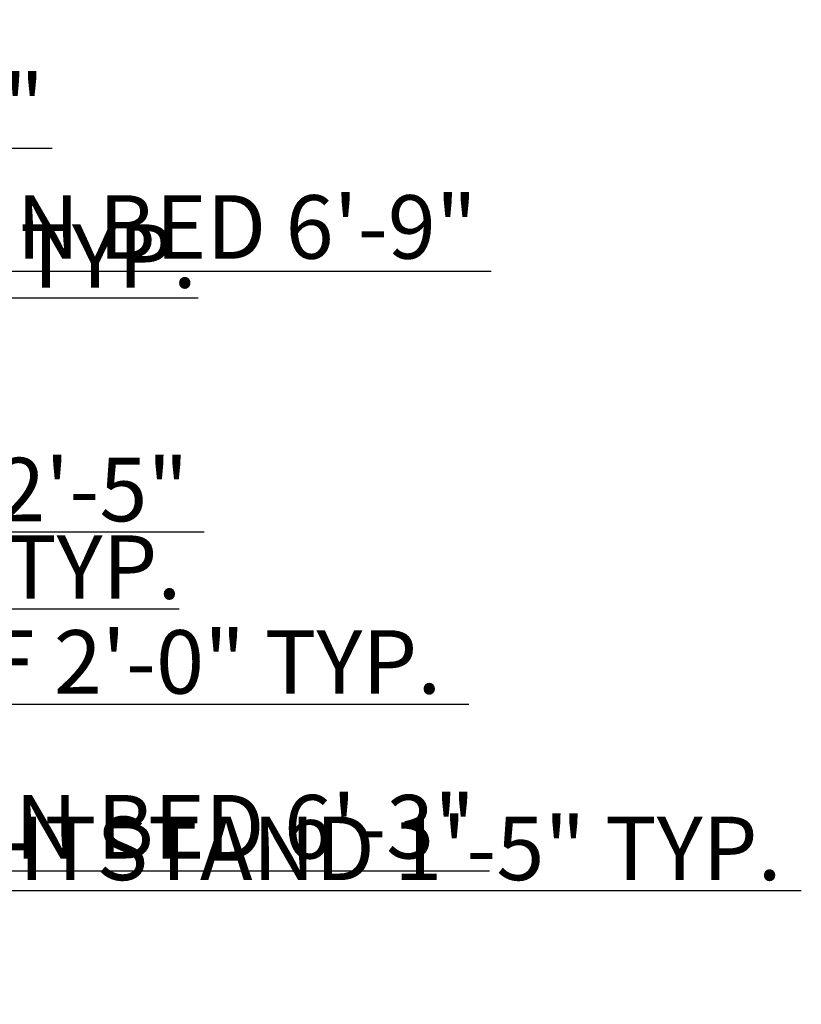
# Model space of a CAD drawing. Units: inches. Extents: x 1102 to 2414, y 295 to 1561.
# Tile 11 of 11: x 1971 to 2414, y 591 to 1150. Entities that reach past the tile are written whole.
import ezdxf

# ---------------------------------------------------------------- set-up
doc = ezdxf.new("R2010")
doc.units = ezdxf.units.IN
doc.layers.add('A-ANNO-DIMS', color=2, linetype='Continuous', lineweight=18)
doc.styles.get("Standard").update_dxf_attribs({"font": 'arial.ttf'})
doc.dimstyles.new('ISO-25', dxfattribs={"dimtxt": 36, "dimasz": 24, "dimexe": 1.25, "dimexo": 0.625, "dimtad": 1, "dimlunit": 4, "dimtxsty": 'Standard', "dimcen": 2.5, "dimadec": 0, "dimazin": 0, "dimtfac": 1, "dimtmove": 0, "dimatfit": 3, "dimfxl": 1, "dimarcsym": 0})

# ---------------------------------------------------------------- blocks, each defined once
blk = doc.blocks.new('*D19')
at = {"layer": 'A-ANNO-DIMS', "color": 0, "lineweight": -2, "transparency": 16777216}
for p, q in [((1765.04, 655.93), (1741.04, 655.93)), ((1789.04, 657.86), (1789.04, 654.68)), ((1789.04, 655.93), (1806.03, 655.93)), ((1806.03, 657.86), (1806.03, 654.68)), ((1830.03, 655.93), (2413.84, 655.93))]:
    blk.add_line(p, q, dxfattribs=at)
at = {"layer": 'A-ANNO-DIMS', "color": 0, "transparency": 16777216}
for points in [[(1765.04, 659.93), (1765.04, 651.93), (1789.04, 655.93)], [(1830.03, 659.93), (1830.03, 651.93), (1806.03, 655.93)]]:
    blk.add_solid(points, dxfattribs=at)
at = {"layer": 'Defpoints', "color": 0, "transparency": 16777216}
for p in [(1789.04, 658.48), (1806.03, 658.48), (1806.03, 655.93)]:
    blk.add_point(p, dxfattribs=at)
at = {"layer": 'A-ANNO-DIMS', "color": 0, "transparency": 16777216, "insert": (2133.94, 675.17), "char_height": 36, "attachment_point": 5}
blk.add_mtext('NIGHTSTAND 1\'-5" TYP.', dxfattribs=at)
blk = doc.blocks.new('*D21')
at = {"layer": 'A-ANNO-DIMS', "color": 0, "lineweight": -2, "transparency": 16777216}
for p, q in [((1731.22, 677.69), (1731.22, 665.84)), ((1806.03, 677.69), (1806.03, 665.84)), ((1755.22, 667.09), (1782.03, 667.09)), ((1806.03, 667.09), (2237.1, 667.09))]:
    blk.add_line(p, q, dxfattribs=at)
at = {"layer": 'A-ANNO-DIMS', "color": 0, "transparency": 16777216}
for points in [[(1755.22, 671.09), (1755.22, 663.09), (1731.22, 667.09)], [(1782.03, 671.09), (1782.03, 663.09), (1806.03, 667.09)]]:
    blk.add_solid(points, dxfattribs=at)
at = {"layer": 'Defpoints', "color": 0, "transparency": 16777216}
for p in [(1731.22, 678.32), (1806.03, 678.32), (1806.03, 667.09)]:
    blk.add_point(p, dxfattribs=at)
at = {"layer": 'A-ANNO-DIMS', "color": 0, "transparency": 16777216, "insert": (2033.56, 687.44), "char_height": 36, "attachment_point": 5}
blk.add_mtext('QUEEN BED 6\'-3"', dxfattribs=at)
blk = doc.blocks.new('*D23')
at = {"layer": 'A-ANNO-DIMS', "color": 0, "lineweight": -2, "transparency": 16777216}
for p, q in [((1725.8, 1018.76), (1725.8, 1005.96)), ((1806.97, 1018.76), (1806.97, 1005.96)), ((1749.8, 1007.21), (1782.97, 1007.21)), ((1806.97, 1007.21), (2238.05, 1007.21))]:
    blk.add_line(p, q, dxfattribs=at)
at = {"layer": 'A-ANNO-DIMS', "color": 0, "transparency": 16777216}
for points in [[(1749.8, 1011.21), (1749.8, 1003.21), (1725.8, 1007.21)], [(1782.97, 1011.21), (1782.97, 1003.21), (1806.97, 1007.21)]]:
    blk.add_solid(points, dxfattribs=at)
at = {"layer": 'Defpoints', "color": 0, "transparency": 16777216}
for p in [(1725.8, 1019.39), (1806.97, 1019.39), (1806.97, 1007.21)]:
    blk.add_point(p, dxfattribs=at)
at = {"layer": 'A-ANNO-DIMS', "color": 0, "transparency": 16777216, "insert": (2034.51, 1027.55), "char_height": 36, "attachment_point": 5}
blk.add_mtext('QUEEN BED 6\'-9"', dxfattribs=at)
blk = doc.blocks.new('*D26')
at = {"layer": 'A-ANNO-DIMS', "color": 0, "lineweight": -2, "transparency": 16777216}
for p, q in [((1750.81, 815.69), (1726.81, 815.69)), ((1774.81, 820.02), (1774.81, 814.44)), ((1774.81, 815.69), (1795.81, 815.69)), ((1795.81, 820.02), (1795.81, 814.44)), ((1819.81, 815.69), (2061.11, 815.69))]:
    blk.add_line(p, q, dxfattribs=at)
at = {"layer": 'A-ANNO-DIMS', "color": 0, "transparency": 16777216}
for points in [[(1750.81, 819.69), (1750.81, 811.69), (1774.81, 815.69)], [(1819.81, 819.69), (1819.81, 811.69), (1795.81, 815.69)]]:
    blk.add_solid(points, dxfattribs=at)
at = {"layer": 'Defpoints', "color": 0, "transparency": 16777216}
for p in [(1774.81, 820.65), (1795.81, 820.65), (1795.81, 815.69)]:
    blk.add_point(p, dxfattribs=at)
at = {"layer": 'A-ANNO-DIMS', "color": 0, "transparency": 16777216, "insert": (1952.46, 834.69), "char_height": 36, "attachment_point": 5}
blk.add_mtext('1\'-9" TYP.', dxfattribs=at)
blk = doc.blocks.new('*D30')
at = {"layer": 'A-ANNO-DIMS', "color": 0, "lineweight": -2, "transparency": 16777216}
for p, q in [((1751.54, 992.03), (1727.54, 992.03)), ((1775.54, 988.38), (1775.54, 993.28)), ((1775.54, 992.03), (1802.54, 992.03)), ((1802.54, 988.38), (1802.54, 993.28)), ((1826.54, 992.03), (2071.85, 992.03))]:
    blk.add_line(p, q, dxfattribs=at)
at = {"layer": 'A-ANNO-DIMS', "color": 0, "transparency": 16777216}
for points in [[(1751.54, 996.03), (1751.54, 988.03), (1775.54, 992.03)], [(1826.54, 996.03), (1826.54, 988.03), (1802.54, 992.03)]]:
    blk.add_solid(points, dxfattribs=at)
at = {"layer": 'Defpoints', "color": 0, "transparency": 16777216}
for p in [(1802.54, 992.03), (1775.54, 987.76), (1802.54, 987.76)]:
    blk.add_point(p, dxfattribs=at)
at = {"layer": 'A-ANNO-DIMS', "color": 0, "transparency": 16777216, "insert": (1961.19, 1011.05), "char_height": 36, "attachment_point": 5}
blk.add_mtext('2\'-3" TYP.', dxfattribs=at)
blk = doc.blocks.new('*D31')
at = {"layer": 'A-ANNO-DIMS', "color": 0, "lineweight": -2, "transparency": 16777216}
for p, q in [((1605.86, 761.66), (1581.86, 761.66)), ((1629.86, 764.63), (1629.86, 760.41)), ((1629.86, 761.66), (1653.86, 761.66)), ((1653.86, 764.63), (1653.86, 760.41)), ((1677.86, 761.66), (2225.36, 761.66))]:
    blk.add_line(p, q, dxfattribs=at)
at = {"layer": 'A-ANNO-DIMS', "color": 0, "transparency": 16777216}
for points in [[(1605.86, 765.66), (1605.86, 757.66), (1629.86, 761.66)], [(1677.86, 765.66), (1677.86, 757.66), (1653.86, 761.66)]]:
    blk.add_solid(points, dxfattribs=at)
at = {"layer": 'Defpoints', "color": 0, "transparency": 16777216}
for p in [(1629.86, 765.26), (1653.86, 765.26), (1653.86, 761.66)]:
    blk.add_point(p, dxfattribs=at)
at = {"layer": 'A-ANNO-DIMS', "color": 0, "transparency": 16777216, "insert": (1963.61, 780.91), "char_height": 36, "attachment_point": 5}
blk.add_mtext('DOOR LEAF 2\'-0" TYP.', dxfattribs=at)
blk = doc.blocks.new('*D33')
at = {"layer": 'A-ANNO-DIMS', "color": 0, "lineweight": -2, "transparency": 16777216}
for p, q in [((1623.16, 1080.7), (1623.16, 1075.57)), ((1653.16, 1080.7), (1653.16, 1075.57)), ((1599.16, 1076.82), (1575.16, 1076.82)), ((1623.16, 1076.82), (1653.16, 1076.82)), ((1677.16, 1076.82), (1989.06, 1076.82))]:
    blk.add_line(p, q, dxfattribs=at)
at = {"layer": 'A-ANNO-DIMS', "color": 0, "transparency": 16777216}
for points in [[(1599.16, 1080.82), (1599.16, 1072.82), (1623.16, 1076.82)], [(1677.16, 1080.82), (1677.16, 1072.82), (1653.16, 1076.82)]]:
    blk.add_solid(points, dxfattribs=at)
at = {"layer": 'Defpoints', "color": 0, "transparency": 16777216}
for p in [(1623.16, 1081.32), (1653.16, 1081.32), (1653.16, 1076.82)]:
    blk.add_point(p, dxfattribs=at)
at = {"layer": 'A-ANNO-DIMS', "color": 0, "transparency": 16777216, "insert": (1845.11, 1096.06), "char_height": 36, "attachment_point": 5}
blk.add_mtext('RANGE 2\'-6"', dxfattribs=at)
blk = doc.blocks.new('*D39')
at = {"layer": 'A-ANNO-DIMS', "color": 0, "lineweight": -2, "transparency": 16777216}
for p, q in [((1623.32, 855.67), (1623.32, 860.64)), ((1652.27, 855.67), (1652.27, 860.64)), ((1599.32, 859.39), (1575.32, 859.39)), ((1623.32, 859.39), (1652.27, 859.39)), ((1676.27, 859.39), (2075.12, 859.39))]:
    blk.add_line(p, q, dxfattribs=at)
at = {"layer": 'A-ANNO-DIMS', "color": 0, "transparency": 16777216}
for points in [[(1599.32, 863.39), (1599.32, 855.39), (1623.32, 859.39)], [(1676.27, 863.39), (1676.27, 855.39), (1652.27, 859.39)]]:
    blk.add_solid(points, dxfattribs=at)
at = {"layer": 'Defpoints', "color": 0, "transparency": 16777216}
for p in [(1623.32, 855.05), (1652.27, 859.39), (1652.27, 855.05)]:
    blk.add_point(p, dxfattribs=at)
at = {"layer": 'A-ANNO-DIMS', "color": 0, "transparency": 16777216, "insert": (1887.69, 878.64), "char_height": 36, "attachment_point": 5}
blk.add_mtext('LOVESEAT 2\'-5"', dxfattribs=at)

msp = doc.modelspace()

# ---------------------------------------------------------------- dimensions: what is measured, and where the dimension line sits
at = {"layer": 'A-ANNO-DIMS'}
for base, p1, p2, text, picture, middle in [((1653.162, 1076.821), (1623.162, 1081.321), (1653.162, 1081.321), 'RANGE <>', '*D33', (1845.112, 1096.06)), ((1806.973, 1007.211), (1725.798, 1019.387), (1806.973, 1019.387), 'QUEEN BED <>', '*D23', (2034.509, 1027.555)), ((1802.544, 992.035), (1775.544, 987.76), (1802.544, 987.76), '<> TYP.', '*D30', (1961.195, 1011.053)), ((1652.268, 859.388), (1623.32, 855.046), (1652.268, 855.046), 'LOVESEAT <>', '*D39', (1887.695, 878.64)), ((1653.864, 761.66), (1629.864, 765.26), (1653.864, 765.26), 'DOOR LEAF <> TYP.', '*D31', (1963.611, 780.911)), ((1795.807, 815.689), (1774.807, 820.646), (1795.807, 820.646), '<> TYP.', '*D26', (1952.457, 834.695)), ((1806.028, 667.095), (1731.225, 678.315), (1806.028, 678.315), 'QUEEN BED <>', '*D21', (2033.565, 687.439)), ((1806.028, 655.933), (1789.038, 658.482), (1806.028, 658.482), 'NIGHTSTAND <> TYP.', '*D19', (2133.936, 675.172))]:
    dim = msp.add_linear_dim(base=base, p1=p1, p2=p2, text=text, dimstyle='ISO-25', override={"dimdec": 1, "dimlfac": 1, "dimrnd": 0, "dimzin": 1, "dimdsep": 46, "dimlunit": 4, "dimfrac": 2}, dxfattribs=at)
    dim.commit()
    dim.dimension.update_dxf_attribs({"geometry": picture, "text_midpoint": middle})

doc.saveas('drawing.dxf')
